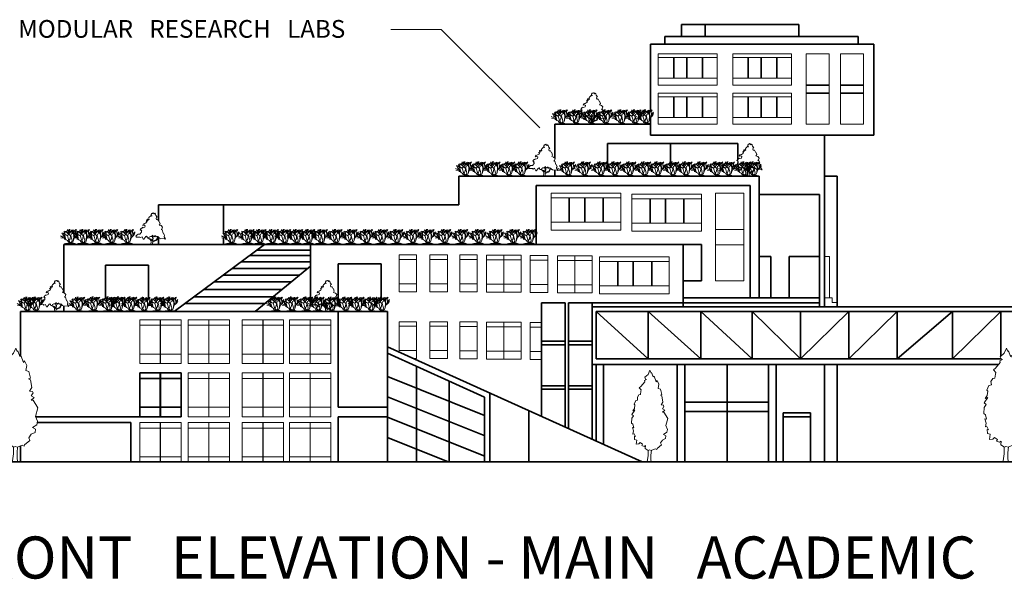
# Model space of a CAD drawing. Units: inches. Extents: x -1080 to 1950, y -1929 to 857.
# Tile 3 of 16: x -622 to -30, y -61 to 275. Entities that reach past the tile are written whole.
import ezdxf

# ---------------------------------------------------------------- set-up
doc = ezdxf.new("R2010")
doc.units = ezdxf.units.IN
doc.header["$MEASUREMENT"] = 0
for name, color, linetype, lineweight in [('A-ANNO-SYMB', 2, 'Continuous', 18), ('A-ANNO-TEXT', 7, 'Continuous', 25), ('A-ELEV', 7, 'Continuous', 35), ('A-GLAZ', 4, 'Continuous', 18), ('L-PLNT', 82, 'Continuous', 13)]:
    doc.layers.add(name, color=color, linetype=linetype, lineweight=lineweight)
doc.styles.get("Standard").update_dxf_attribs({"font": 'arial.ttf'})

# ---------------------------------------------------------------- blocks, each defined once
blk = doc.blocks.new('*U5')
blk.add_lwpolyline([(-2.754, 191.699), (-6.78, 182.851), (-13.682, 176.953), (-11.956, 173.266), (-9.656, 172.529), (-14.257, 170.317), (-13.682, 167.368), (-21.733, 157.783), (-25.184, 154.834), (-21.158, 150.41), (-21.733, 147.461), (-22.884, 140.825), (-26.334, 140.087), (-29.21, 134.926), (-28.635, 129.028), (-32.661, 128.291), (-36.111, 120.18), (-34.386, 118.706), (-35.536, 111.333), (-38.987, 106.171), (-34.386, 107.646), (-40.712, 98.798), (-37.261, 95.849), (-40.712, 90.688), (-41.287, 80.366), (-38.412, 78.154), (-36.686, 70.781), (-39.562, 71.518), (-37.261, 64.145), (-38.412, 57.509), (-36.111, 58.247), (-33.236, 52.348), (-35.536, 53.086), (-34.961, 46.45), (-30.36, 44.975), (-31.51, 36.128), (-26.334, 36.865), (-23.459, 39.814), (-18.283, 36.128), (-20.008, 33.178), (-14.832, 31.704), (-11.956, 33.178), (-12.531, 27.28), (-6.205, 22.856), (-3.905, 24.331), (0.121, 22.856), (8.173, 26.543), (11.624, 25.068), (12.199, 27.28), (21.4, 34.653), (19.675, 39.077), (23.701, 44.975), (30.027, 47.924), (30.602, 53.823), (25.426, 56.772), (32.903, 61.196), (34.053, 67.094), (30.602, 75.205), (34.628, 89.951), (26.576, 103.222), (23.701, 103.222), (28.302, 107.646), (23.701, 110.595), (26.576, 115.756), (25.426, 117.968), (20.825, 118.706), (24.276, 124.604), (22.551, 137.876), (19.1, 139.35), (22.551, 140.825), (19.675, 151.884), (14.499, 153.359), (16.224, 162.207), (12.199, 170.317), (10.473, 167.368), (5.872, 179.165), (4.147, 177.69), (0.696, 187.275), (-0.454, 185.8)], close=True)
for points in [[(-6.813, 23.669), (-6.813, 11.669), (-8.627, 0)], [(0.387, 23.669), (-0.576, 13.271), (-0.576, 3.686), (0, 0)]]:
    blk.add_lwpolyline(points)
blk = doc.blocks.new('*U2')
for points in [[(22.0124, 137.721), (18.5475, 141.5624), (15.5282, 138.2446), (13.8028, 139.3505), (13.3714, 142.1153), (11.2148, 143.2214), (8.1954, 140.4564), (4.7447, 141.0094), (2.1567, 136.0326), (2.1567, 131.6088), (5.6074, 129.9499), (3.0193, 128.2909), (0.4313, 130.5029), (-6.9015, 123.3141), (-6.9015, 121.6552), (-9.9208, 119.9963), (-9.0581, 118.3373), (-6.9015, 115.0195), (-10.7835, 112.2546), (-14.6656, 115.0195), (-16.8222, 114.4665), (-17.6849, 112.2546), (-14.6656, 111.7016), (-14.2342, 107.2778), (-17.6065, 107.8307), (-21.5669, 103.9599), (-17.2536, 103.4069), (-18.9789, 97.8771), (-22.8609, 97.3241), (-27.1743, 94.5593), (-32.3504, 91.7944), (-32.7817, 94.0063), (-36.6638, 85.7116), (-29.7624, 87.3705), (-25.449, 84.6056), (-26.743, 77.9699), (-34.507, 75.205), (-37.9578, 77.4169), (-39.2518, 74.099), (-42.2711, 73.5461), (-44.8592, 70.2282), (-47.8786, 66.3574), (-43.9965, 63.0395), (-41.4085, 64.6985), (-44.3346, 59.8898), (-42.2089, 60.1377), (-42.5159, 55.7849), (-49.6039, 46.4502), (-58.2307, 45.8972), (-62.1127, 43.6853), (-68.5828, 36.4966), (-65.9947, 32.0727), (-50.0352, 32.6257), (-47.0159, 30.4138), (-39.6831, 33.7317), (-34.507, 22.6721), (-32.3504, 22.6721), (-22.4296, 34.8376), (-19.4102, 36.4966), (-17.2536, 33.7317), (-17.2536, 29.8608), (-13.8028, 28.7549), (-9.0581, 28.7549), (-7.3328, 32.6257), (-1.7254, 35.3906), (3.8821, 35.9436), (6.4701, 38.1555), (6.9014, 38.7085), (8.1954, 41.4734), (9.9208, 40.3674), (11.2148, 35.9436), (14.2341, 37.6025), (15.0968, 36.4966), (15.9595, 33.7317), (18.9789, 38.7085), (21.9982, 38.7085), (23.2922, 36.4966), (21.9982, 34.2847), (25.4489, 35.3906), (26.743, 33.7317), (29.7623, 35.9436), (32.7817, 34.8376), (38.8204, 28.7549), (41.4084, 27.6489), (43.5651, 25.437), (61.6813, 27.0959), (65.132, 23.7781), (67.7201, 24.884), (60.8186, 33.7317), (60.3873, 37.0495), (62.544, 40.3674), (58.662, 50.874), (56.5053, 50.874), (52.1919, 66.3574), (47.8785, 66.9103), (50.4665, 69.1222), (53.9172, 77.9699), (47.0158, 85.1586), (38.3891, 87.9235), (42.2711, 94.0063)], [(42.2711, 94.0063), (38.8204, 104.5129), (36.6637, 104.5129), (32.3503, 113.9135), (29.7623, 113.3605), (26.743, 113.3605), (24.5862, 117.7844), (25.8802, 123.8671), (29.331, 123.8671), (22.8609, 131.6088), (21.9982, 137.6916)], [(-12.9401, 28.7549), (-2.588, 22.1191), (0.8626, 17.6953), (1.7253, 11.6125), (0, 0)], [(-9.9208, 28.2019), (0, 23.2251), (3.4507, 19.9072), (4.7447, 15.4834), (8.6267, 27.0959), (6.4701, 37.6025)], [(34.5071, 33.1787), (27.1743, 18.2483), (9.0581, 10.5066), (7.7641, 3.8708), (8.1954, 0)], [(8.1954, 40.3674), (11.2148, 27.6489), (8.1954, 13.8245), (24.5862, 19.9072), (32.7817, 34.2847)]]:
    blk.add_lwpolyline(points)
blk = doc.blocks.new('*U6')
for p, q in [((-463.296, 280.416), (-552.577, 423.037)), ((-329.184, 316.992), (-499.872, 414.528)), ((-426.72, 414.528), (-475.488, 475.488)), ((-377.952, 463.296), (-451.104, 487.68)), ((-426.72, 414.528), (-390.144, 499.872)), ((-426.72, 316.992), (-426.72, 414.528)), ((-377.952, 463.296), (-329.184, 524.256)), ((-207.264, 304.8), (-377.952, 463.296)), ((-338.455, 424.7896), (-290.3982, 464.5406)), ((-329.184, 316.992), (-207.264, 451.104)), ((-316.7634, 502.285), (-327.6092, 559.9176)), ((-296.5958, 484.4034), (-316.7634, 502.285)), ((-286.512, 498.3226), (-307.4416, 538.0736)), ((-305.8922, 396.9512), (-302.7934, 478.4344)), ((-304.3428, 426.7708), (-268.7066, 458.5716)), ((-302.7934, 478.4344), (-270.256, 518.1854)), ((-290.3982, 464.5406), (-265.6078, 577.8246)), ((-268.7066, 458.5716), (-250.0884, 500.3038)), ((-207.264, 451.104), (-268.224, 548.64)), ((-240.792, 502.285), (-228.3968, 573.8368)), ((-182.88, 499.872), (-219.456, 512.064)), ((-207.264, 451.104), (-134.112, 487.68)), ((-182.88, 499.872), (-158.496, 536.448)), ((-121.92, 414.528), (-182.88, 499.872)), ((-182.88, 377.952), (-97.536, 426.72)), ((-129.1844, 450.6214), (-140.0302, 542.036)), ((-134.112, 487.68), (-97.536, 548.64)), ((-85.7758, 389.001), (-129.1844, 452.6026)), ((-73.152, 329.184), (-109.728, 499.872)), ((-97.536, 426.72), (-24.384, 524.256)), ((-85.7758, 472.4908), (-73.3552, 548.005)), ((-70.2564, 426.7708), (-85.7758, 472.4908)), ((-73.152, 402.336), (-60.96, 512.064)), ((-24.384, 268.224), (-73.152, 402.336)), ((-12.9032, 555.9552), (-2.0574, 522.1732)), ((-5.1562, 486.3846), (2.5908, 542.036)), ((8.7884, 335.3562), (-5.1562, 486.3846)), ((-3.6068, 492.3536), (14.986, 518.1854)), ((-0.508, 508.254), (22.7584, 536.067)), ((1.0414, 526.1356), (35.1536, 559.9176)), ((2.5908, 542.036), (21.209, 555.9552)), ((8.7884, 335.3562), (33.6042, 412.8516)), ((24.384, 304.8), (36.576, 390.144)), ((33.6042, 412.8516), (92.5068, 464.5406)), ((36.576, 390.144), (73.152, 438.912)), ((48.768, 341.376), (60.96, 390.144)), ((60.96, 390.144), (85.344, 414.528)), ((-451.104, 219.456), (-601.0402, 303.8094)), ((-451.104, 219.456), (-587.4512, 234.2388)), ((-463.296, 280.416), (-512.064, 292.608)), ((-353.568, 316.992), (-487.68, 377.952)), ((-402.336, 207.264), (-463.296, 280.416)), ((-414.528, 182.88), (-463.296, 182.88)), ((-426.72, 316.992), (-451.104, 329.184)), ((-377.952, 146.304), (-451.104, 219.456)), ((-402.336, 12.192), (-451.104, 0)), ((-402.336, 207.264), (-426.72, 316.992)), ((-377.952, 146.304), (-402.336, 207.264)), ((-341.376, 12.192), (-402.336, 12.192)), ((-329.184, 121.92), (-377.952, 146.304)), ((-329.184, 316.992), (-353.568, 316.992)), ((-243.84, 24.384), (-341.376, 12.192)), ((-268.224, 109.728), (-329.184, 316.992)), ((-292.608, 60.96), (-329.184, 121.92)), ((-243.84, 24.384), (-329.184, 0)), ((-219.456, 24.384), (-292.608, 60.96)), ((-268.224, 109.728), (-219.456, 195.072)), ((-219.456, 48.768), (-268.224, 109.728)), ((-243.84, 24.384), (-195.072, 24.384)), ((-219.456, 195.072), (-207.264, 304.8)), ((-219.456, 24.384), (-109.728, 73.152)), ((-219.456, 24.384), (-158.496, 73.152)), ((-219.456, 24.384), (-219.456, 48.768)), ((-219.456, 24.384), (-73.152, 24.384)), ((-195.072, 316.992), (-182.88, 377.952)), ((-170.688, 219.456), (-195.072, 316.992)), ((-195.072, 24.384), (-158.496, 12.192)), ((-146.304, 134.112), (-170.688, 219.456)), ((-158.496, 73.152), (-146.304, 134.112)), ((-158.496, 12.192), (-85.344, 0)), ((-109.728, 73.152), (-48.768, 243.84)), ((-85.344, 134.112), (-73.152, 329.184)), ((-73.152, 24.384), (0, 0)), ((-48.768, 243.84), (24.384, 304.8)), ((-12.192, 274.32), (8.7884, 335.3562)), ((24.384, 304.8), (73.152, 377.952))]:
    blk.add_line(p, q)
blk = doc.blocks.new('*U4')
for points in [[(559.11496, 3498.1134), (471.1065, 3595.68496), (394.41628, 3511.41284), (350.59112, 3539.5027), (339.63356, 3609.72862), (284.85592, 3637.82356), (208.16316, 3567.59256), (120.51538, 3581.63876), (54.78018, 3455.22804), (54.78018, 3342.86352), (142.42796, 3300.72746), (76.69022, 3258.58886), (10.95502, 3314.77366), (-175.2981, 3132.17814), (-175.2981, 3090.04208), (-251.98832, 3047.90602), (-230.07574, 3005.76742), (-175.2981, 2921.4953), (-273.9009, 2851.26684), (-372.50624, 2921.4953), (-427.28388, 2907.4491), (-449.19646, 2851.26684), (-372.50624, 2837.22064), (-361.54868, 2724.85612), (-447.2051, 2738.89978), (-547.79926, 2640.58146), (-438.24144, 2626.53526), (-482.06406, 2486.07834), (-580.66686, 2472.03214), (-690.22722, 2401.80622), (-821.70016, 2331.57776), (-832.65518, 2387.76002), (-931.26052, 2177.07464), (-755.96496, 2219.2107), (-646.4046, 2148.98224), (-679.2722, 1980.43546), (-876.4778, 1910.207), (-964.12812, 1966.38926), (-996.99572, 1882.1146), (-1073.68594, 1868.07094), (-1139.42368, 1783.79628), (-1216.11644, 1685.47796), (-1117.5111, 1601.2033), (-1051.7759, 1643.3419), (-1126.09884, 1521.20092), (-1072.10606, 1527.49758), (-1079.90386, 1416.93646), (-1259.93906, 1179.83508), (-1479.05978, 1165.78888), (-1577.66258, 1109.60662), (-1742.00312, 927.01364), (-1676.26538, 814.64658), (-1270.89408, 828.69278), (-1194.20386, 772.51052), (-1007.95074, 856.78518), (-876.4778, 575.87134), (-821.70016, 575.87134), (-569.71184, 884.87504), (-493.01908, 927.01364), (-438.24144, 856.78518), (-438.24144, 758.46432), (-350.59112, 730.37446), (-230.07574, 730.37446), (-186.25312, 828.69278), (-43.82516, 898.92124), (98.60534, 912.96744), (164.34054, 969.1497), (175.29556, 983.1959), (208.16316, 1053.42436), (251.98832, 1025.33196), (284.85592, 912.96744), (361.54614, 955.1035), (383.45872, 927.01364), (405.3713, 856.78518), (482.06406, 983.1959), (558.75428, 983.1959), (591.62188, 927.01364), (558.75428, 870.83138), (646.40206, 898.92124), (679.2722, 856.78518), (755.96242, 912.96744), (832.65518, 884.87504), (986.03816, 730.37446), (1051.77336, 702.28206), (1106.55354, 646.0998), (1566.70502, 688.23586), (1654.3528, 603.96374), (1720.09054, 632.0536), (1544.79244, 856.78518), (1533.83742, 941.0573), (1588.6176, 1025.33196), (1490.0148, 1292.1996), (1435.23462, 1292.1996), (1325.67426, 1685.47796), (1216.1139, 1699.52162), (1281.8491, 1755.70388), (1369.49688, 1980.43546), (1194.20132, 2163.02844), (975.08314, 2233.2569), (1073.68594, 2387.76002)], [(1073.68594, 2387.76002), (986.03816, 2654.62766), (931.25798, 2654.62766), (821.69762, 2893.4029), (755.96242, 2879.3567), (679.2722, 2879.3567), (624.48948, 2991.72376), (657.35708, 3146.22434), (745.0074, 3146.22434), (580.66686, 3342.86352), (558.75428, 3497.36664)], [(-328.67854, 730.37446), (-65.7352, 561.82514), (21.91004, 449.46062), (43.82262, 294.9575), (0, 0)], [(-251.98832, 716.32826), (0, 589.91754), (87.64778, 505.64288), (120.51538, 393.27836), (219.11818, 688.23586), (164.34054, 955.1035)], [(876.48034, 842.73898), (690.22722, 463.50682), (230.07574, 266.86764), (197.20814, 98.31832), (208.16316, 0)], [(208.16316, 1025.33196), (284.85592, 702.28206), (208.16316, 351.1423), (624.48948, 505.64288), (832.65518, 870.83138)]]:
    blk.add_lwpolyline(points)
blk = doc.blocks.new('WIN-TYPE-A')
for p, q in [((12.45, 26.32), (0, 26.32)), ((0, 26.32), (0, 23.06)), ((24.78, 26.32), (12.34, 26.32)), ((12.34, 26.32), (12.34, 23.06)), ((12.45, 26.32), (12.45, 23.06)), ((24.78, 26.32), (24.78, 23.06)), ((0, 23.06), (0, 5.73)), ((0, 23.06), (12.45, 23.06)), ((12.34, 23.06), (12.34, 5.73)), ((12.34, 23.06), (24.78, 23.06)), ((12.45, 5.73), (12.45, 23.06)), ((24.78, 5.73), (24.78, 23.06)), ((0, 5.73), (12.45, 5.73)), ((0, 5.73), (0, 0)), ((0, 0), (12.45, 0)), ((12.34, 5.73), (24.78, 5.73)), ((12.34, 5.73), (12.34, 0)), ((12.34, 0), (24.78, 0)), ((12.45, 0), (12.45, 5.73)), ((24.78, 0), (24.78, 5.73))]:
    blk.add_line(p, q)
blk = doc.blocks.new('WIN-TYPE-B')
for p, q in [((10.5, 22.21), (0, 22.21)), ((0, 22.21), (0, 19.45)), ((0, 19.45), (0, 4.84)), ((0, 19.45), (10.5, 19.45)), ((20.91, 22.21), (10.41, 22.21)), ((10.41, 22.21), (10.41, 19.45)), ((10.41, 19.45), (10.41, 4.84)), ((10.41, 19.45), (20.91, 19.45)), ((10.5, 22.21), (10.5, 19.45)), ((10.5, 4.84), (10.5, 19.45)), ((20.91, 22.21), (20.91, 19.45)), ((20.91, 4.84), (20.91, 19.45)), ((0, 4.84), (10.5, 4.84)), ((0, 4.84), (0, 0)), ((0, 0), (10.5, 0)), ((10.41, 4.84), (20.91, 4.84)), ((10.41, 4.84), (10.41, 0)), ((10.41, 0), (20.91, 0)), ((10.5, 0), (10.5, 4.84)), ((20.91, 0), (20.91, 4.84))]:
    blk.add_line(p, q)
blk = doc.blocks.new('WIN-TYPE-C')
for p, q in [((12.45, 23.64), (0, 23.64)), ((0, 23.64), (0, 20.37)), ((0, 20.37), (0, 3.04)), ((0, 20.37), (12.45, 20.37)), ((24.78, 23.64), (12.34, 23.64)), ((12.34, 23.64), (12.34, 20.37)), ((12.34, 20.37), (12.34, 3.04)), ((12.34, 20.37), (24.78, 20.37)), ((12.45, 23.64), (12.45, 20.37)), ((12.45, 3.04), (12.45, 20.37)), ((24.78, 23.64), (24.78, 20.37)), ((24.78, 3.04), (24.78, 20.37)), ((0, 3.04), (12.45, 3.04)), ((0, 3.04), (0, 0)), ((12.34, 3.04), (24.78, 3.04)), ((12.34, 3.04), (12.34, 0)), ((12.45, 0), (12.45, 3.04)), ((24.78, 0), (24.78, 3.04))]:
    blk.add_line(p, q)
blk = doc.blocks.new('WIN-TYPE-E')
for p, q in [((10.5, 22.21), (0, 22.21)), ((0, 22.21), (0, 19.45)), ((0, 19.45), (0, 4.84)), ((0, 19.45), (10.5, 19.45)), ((10.5, 22.21), (10.5, 19.45)), ((10.5, 4.84), (10.5, 19.45)), ((0, 4.84), (10.5, 4.84)), ((0, 4.84), (0, 0)), ((0, 0), (10.5, 0)), ((10.5, 0), (10.5, 4.84))]:
    blk.add_line(p, q)
blk = doc.blocks.new('WIN-TYPE-G')
for p, q in [((0, 19.45), (0, 22.21)), ((0, 22.21), (41.85, 22.21)), ((0, 19.45), (0, 4.84)), ((41.85, 19.45), (0, 19.45)), ((41.85, 22.21), (41.85, 19.45)), ((41.85, 4.84), (41.85, 19.45)), ((0, 4.84), (41.85, 4.84)), ((0, 4.84), (0, 0)), ((41.85, 0), (41.85, 4.84)), ((0, 0), (41.85, 0))]:
    blk.add_line(p, q)
blk = doc.blocks.new('WIN-TYPE-H')
for p, q in [((0, 16.47), (0, 18.8)), ((0, 18.8), (35.42, 18.8)), ((35.42, 18.8), (35.42, 16.47)), ((0, 16.47), (0, 4.09)), ((35.42, 16.47), (0, 16.47)), ((35.42, 4.09), (35.42, 16.47)), ((0, 4.09), (35.42, 4.09)), ((0, 4.09), (0, 0)), ((35.42, 0), (35.42, 4.09)), ((0, 0), (35.42, 0))]:
    blk.add_line(p, q)
blk = doc.blocks.new('WIN-TYPE-N')
for p, q in [((0, 52.66), (17.07, 52.66)), ((0, 30.88), (0, 52.66)), ((17.07, 52.66), (17.07, 30.88)), ((17.07, 30.88), (0, 30.88)), ((0, 30.88), (0, 21.78)), ((17.07, 30.88), (17.07, 21.78)), ((0, 21.78), (17.07, 21.78)), ((0, 0), (0, 21.78)), ((17.07, 21.78), (17.07, 0)), ((17.07, 0), (0, 0))]:
    blk.add_line(p, q)
blk = doc.blocks.new('WIN-TYPE-P')
for p, q in [((10.5, 22.21), (0, 22.21)), ((0, 22.21), (0, 19.45)), ((0, 19.45), (0, 4.84)), ((0, 19.45), (10.5, 19.45)), ((10.5, 22.21), (10.5, 19.45)), ((10.5, 4.84), (10.5, 19.45)), ((0, 4.84), (10.5, 4.84)), ((0, 4.84), (0, 3.89)), ((8.62, 0), (10.5, 0)), ((10.5, 0), (10.5, 4.84))]:
    blk.add_line(p, q)
blk = doc.blocks.new('PANEL-A')
for p, q in [((0, 42.42), (0, 0)), ((13.76, 42.42), (0, 42.42)), ((13.76, 0), (13.76, 42.42)), ((0, 0), (13.76, 0))]:
    blk.add_line(p, q)
blk = doc.blocks.new('WIN-TYPE-R')
for p, q in [((6.66, 22.21), (0, 22.21)), ((0, 22.21), (0, 19.45)), ((0, 19.45), (0, 4.84)), ((0, 19.45), (6.66, 19.45)), ((0, 4.84), (6.66, 4.84)), ((0, 4.84), (0, 0)), ((0, 0), (6.66, 0))]:
    blk.add_line(p, q)
blk = doc.blocks.new('WIN-TYPE-S')
for p, q in [((0, 27.66), (3.06, 27.66)), ((3.06, 27.66), (3.06, 2.78)), ((3.06, 2.78), (0, 2.78)), ((3.06, 2.78), (4.6, 2.78)), ((4.6, 2.78), (4.6, 0)), ((4.6, 0), (7.75, 0))]:
    blk.add_line(p, q)

msp = doc.modelspace()

# ---------------------------------------------------------------- linework, layer by layer
at = {"layer": 'A-ANNO-SYMB'}
for q in [(-398.58, 268.75), (-308.98, 209.71)]:
    msp.add_line((-368.35, 268.75), q, dxfattribs=at)
at = {"layer": 'A-ELEV'}
for p, q in [((-223.9, 269.6), (-223.9, 271.66)), ((-223.9, 271.66), (-153.32, 271.66)), ((-223.9, 264.54), (-223.9, 269.6)), ((-209.57, 264.54), (-209.57, 271.66)), ((-153.32, 271.66), (-153.32, 264.54)), ((-233.84, 260.04), (-233.84, 264.54)), ((-233.84, 264.54), (-117.77, 264.54)), ((-117.77, 264.54), (-117.77, 260.04)), ((-242.4, 250.46), (-242.4, 260.04)), ((-242.4, 260.04), (-112.68, 260.04)), ((-112.68, 260.04), (-108.18, 260.04)), ((-108.18, 260.04), (-108.18, 210.83)), ((-242.4, 234.12), (-242.4, 250.46)), ((-228.5, 251.89), (-228.5, 239.51)), ((-220.66, 251.89), (-220.66, 239.51)), ((-211.25, 251.89), (-211.25, 239.51)), ((-183.82, 251.89), (-183.82, 239.51)), ((-175.98, 251.89), (-175.98, 239.51)), ((-166.57, 251.89), (-166.57, 239.51)), ((-242.4, 234.12), (-242.4, 219.88)), ((-148.84, 235.42), (-135.08, 235.42)), ((-128.29, 235.42), (-114.53, 235.42)), ((-228.5, 228.27), (-228.5, 215.89)), ((-220.66, 228.27), (-220.66, 215.89)), ((-211.25, 228.27), (-211.25, 215.89)), ((-183.82, 228.27), (-183.82, 215.89)), ((-175.98, 228.27), (-175.98, 215.89)), ((-166.57, 228.27), (-166.57, 215.89)), ((-148.84, 230.6), (-135.08, 230.6)), ((-128.29, 230.6), (-114.53, 230.6)), ((-242.4, 216.14), (-242.4, 206.68)), ((-242.4, 211.8), (-299.96, 211.8)), ((-299.96, 211.8), (-299.96, 191.39)), ((-108.18, 205.21), (-108.18, 210.83)), ((-242.4, 205.21), (-242.4, 206.68)), ((-144.09, 205.21), (-242.4, 205.21)), ((-144.09, 205.21), (-108.18, 205.21)), ((-137.95, 205.21), (-137.95, 102.28)), ((-268.41, 187.18), (-268.41, 200.27)), ((-268.41, 200.27), (-190.05, 200.27)), ((-230.41, 200.27), (-230.41, 186.07)), ((-190.05, 200.27), (-190.05, 190.71)), ((-299.96, 184.41), (-299.96, 180.63)), ((-268.41, 184.1), (-268.41, 185.92)), ((-357.6, 180.63), (-357.6, 163.4)), ((-177.27, 180.63), (-357.6, 180.63)), ((-230.41, 180.95), (-230.41, 180.63)), ((-189.87, 180.68), (-189.87, 180.63)), ((-177.27, 180.63), (-177.27, 107.59)), ((-137.95, 180.63), (-130.2, 180.63)), ((-130.2, 180.63), (-130.2, 102.28)), ((-182.61, 175.14), (-311.15, 175.14)), ((-311.15, 175.14), (-311.15, 146.63)), ((-182.61, 175.14), (-182.61, 107.59)), ((-291.28, 167.62), (-291.28, 153)), ((-282.01, 167.62), (-282.01, 153)), ((-270.9, 167.62), (-270.9, 153)), ((-242.75, 167.07), (-242.75, 152.45)), ((-233.49, 167.07), (-233.49, 152.45)), ((-222.38, 167.07), (-222.38, 152.45)), ((-177.27, 169.72), (-140.99, 169.72)), ((-140.99, 169.72), (-140.99, 102.28)), ((-538.13, 163.4), (-538.13, 153.85)), ((-499.1, 163.4), (-538.13, 163.4)), ((-357.6, 163.4), (-500.54, 163.4)), ((-499.1, 163.4), (-499.1, 145.94)), ((-499.1, 145.94), (-499.1, 163.4)), ((-538.13, 143.98), (-538.13, 139.7)), ((-538.13, 142.55), (-538.13, 140.7)), ((-499.1, 143.57), (-499.1, 139.7)), ((-499.1, 139.7), (-499.1, 143.57)), ((-311.15, 145.47), (-311.15, 139.7)), ((-311.15, 139.7), (-595.05, 139.7)), ((-595.05, 139.7), (-595.05, 110.56)), ((-474.45, 139.7), (-528.73, 99.4)), ((-479.2, 136.17), (-446.74, 136.17)), ((-446.74, 104.8), (-446.74, 139.7)), ((-222.88, 139.7), (-311.15, 139.7)), ((-222.88, 107.59), (-222.88, 139.7)), ((-222.88, 139.7), (-211.87, 139.7)), ((-211.87, 139.7), (-211.87, 117.73)), ((-483.5, 132.98), (-446.74, 132.98)), ((-170.17, 132.47), (-177.27, 132.47)), ((-170.17, 132.47), (-170.17, 107.59)), ((-140.99, 132.47), (-159.06, 132.47)), ((-159.06, 132.47), (-159.06, 107.59)), ((-544.08, 127.31), (-569.96, 127.31)), ((-569.96, 127.31), (-569.96, 107.83)), ((-544.08, 107.26), (-544.08, 127.31)), ((-493.85, 125.3), (-448.32, 125.3)), ((-488.44, 129.31), (-446.74, 129.31)), ((-446.74, 126.59), (-480.05, 99.4)), ((-404.41, 127.96), (-430.29, 127.96)), ((-430.29, 127.96), (-430.29, 105.94)), ((-404.41, 127.96), (-404.41, 105.75)), ((-262.14, 129.43), (-262.14, 114.82)), ((-252.87, 129.43), (-252.87, 114.82)), ((-241.76, 129.43), (-241.76, 114.82)), ((-499.47, 121.13), (-453.43, 121.13)), ((-510.93, 112.62), (-463.85, 112.62)), ((-504.84, 117.14), (-458.32, 117.14)), ((-211.87, 117.73), (-222.88, 117.73)), ((-516.9, 108.19), (-469.28, 108.19)), ((-182.61, 107.59), (-222.88, 107.59)), ((-222.88, 107.59), (-222.88, 102.28)), ((-222.88, 107.59), (-140.99, 107.59)), ((-595.05, 102.6), (-595.05, 99.4)), ((-569.96, 106.21), (-569.96, 105.86)), ((-569.96, 104.47), (-569.96, 104.15)), ((-544.08, 103.03), (-544.08, 103.83)), ((-522.4, 104.1), (-474.29, 104.1)), ((-308.06, 104.57), (-308.06, 102.28)), ((-293.75, 104.57), (-308.06, 104.57)), ((-308.06, 102.28), (-308.06, 36.38)), ((-293.75, 29.92), (-293.75, 104.57)), ((-222.88, 104.57), (-291.77, 104.57)), ((-291.77, 29.03), (-291.77, 104.57)), ((-277.64, 22.66), (-277.64, 104.57)), ((-222.88, 102.28), (-277.64, 102.28)), ((-222.88, 104.57), (-140.99, 104.57)), ((-222.88, 102.28), (-137.95, 102.28)), ((-123.32, 102.28), (-177.27, 102.28)), ((-123.32, 102.28), (2.16, 102.28)), ((-621.1, 72.79), (-621.1, 99.4)), ((-621.1, 99.4), (-400.95, 99.4)), ((-544.08, 99.4), (-544.08, 99.5)), ((-446.74, 99.4), (-446.74, 99.82)), ((-430.29, 99.4), (-430.29, 41.92)), ((-400.48, 99.4), (-409.25, 99.4)), ((-404.41, 100.02), (-404.41, 99.85)), ((-400.48, 99.4), (-400.95, 99.4)), ((-400.48, 99.4), (-400.48, 9.02)), ((-222.88, 99.4), (-275.18, 99.4)), ((-275.18, 99.4), (-275.18, 70.95)), ((-275.18, 99.4), (-243.84, 70.95)), ((-243.84, 99.4), (-243.84, 70.95)), ((-243.84, 99.4), (-212.24, 70.95)), ((-126.4, 99.4), (-222.88, 99.4)), ((-212.24, 99.4), (-212.24, 70.95)), ((-212.24, 99.4), (-181.47, 70.95)), ((-181.47, 99.4), (-181.47, 70.95)), ((-181.47, 99.4), (-152.43, 70.95)), ((-152.43, 99.4), (-152.43, 70.95)), ((-123.32, 99.4), (-152.43, 70.95)), ((1.28, 99.4), (-126.4, 99.4)), ((-123.32, 99.4), (-123.32, 70.95)), ((-94.28, 99.4), (-123.32, 70.95)), ((-94.28, 99.4), (-94.28, 70.95)), ((-60.92, 99.4), (-94.28, 70.95)), ((-60.92, 99.4), (-60.92, 70.95)), ((-31.87, 99.4), (-60.92, 70.95)), ((-31.87, 99.4), (-31.87, 72.61)), ((-400.48, 78.07), (-247.42, 9.02)), ((-308.06, 81.48), (-293.75, 81.48)), ((-308.06, 79.29), (-293.75, 79.29)), ((-291.77, 81.48), (-277.64, 81.48)), ((-291.77, 79.29), (-277.64, 79.29)), ((-400.48, 74.27), (-342.32, 47.95)), ((-31.87, 71.12), (-31.87, 70.95)), ((-383.06, 66.39), (-383.06, 9.02)), ((-112.28, 67.56), (-277.64, 67.56)), ((-123.32, 70.95), (-275.18, 70.95)), ((-275.18, 67.56), (-275.18, 25.36)), ((-270.65, 67.56), (-270.65, 19.5)), ((-226.43, 67.56), (-226.43, 9.02)), ((-221.76, 67.56), (-221.76, 9.02)), ((-196.36, 67.56), (-196.36, 9.02)), ((-171.52, 67.56), (-171.52, 9.02)), ((-166.86, 67.56), (-166.86, 9.02)), ((-137.95, 67.56), (-137.95, 9.02)), ((-130.2, 67.56), (-130.2, 9.02)), ((-31.79, 70.95), (-123.32, 70.95)), ((-33.42, 67.56), (-112.28, 67.56)), ((-536.96, 62.51), (-549.41, 62.51)), ((-549.41, 62.51), (-549.41, 59.24)), ((-549.41, 59.24), (-549.41, 41.92)), ((-549.41, 59.24), (-536.96, 59.24)), ((-524.62, 62.51), (-537.07, 62.51)), ((-537.07, 62.51), (-537.07, 59.24)), ((-537.07, 59.24), (-537.07, 41.92)), ((-537.07, 59.24), (-524.62, 59.24)), ((-536.96, 62.51), (-536.96, 59.24)), ((-536.96, 41.92), (-536.96, 59.24)), ((-524.62, 62.51), (-524.62, 59.24)), ((-524.62, 41.92), (-524.62, 59.24)), ((-400.48, 60.25), (-342.32, 36.88)), ((-363.57, 57.57), (-363.57, 9.02)), ((-308.06, 54.7), (-293.75, 54.7)), ((-291.77, 54.7), (-277.64, 54.7)), ((-400.51, 48.23), (-342.36, 24.86)), ((-342.32, 51.98), (-342.32, 51.84)), ((-342.32, 47.95), (-342.32, 9.02)), ((-339.02, 50.35), (-339.02, 9.02)), ((-308.06, 52.64), (-293.75, 52.64)), ((-291.77, 52.64), (-277.64, 52.64)), ((-549.41, 41.92), (-536.96, 41.92)), ((-549.41, 41.92), (-549.41, 36.18)), ((-537.07, 41.92), (-524.62, 41.92)), ((-537.07, 41.92), (-537.07, 36.18)), ((-536.96, 36.18), (-536.96, 41.92)), ((-524.62, 36.18), (-524.62, 41.92)), ((-430.29, 41.92), (-400.48, 41.92)), ((-221.76, 44.86), (-171.52, 44.86)), ((-554.75, 36.18), (-612.12, 36.18)), ((-554.75, 36.18), (-549.41, 36.18)), ((-549.41, 36.18), (-536.96, 36.18)), ((-537.07, 36.18), (-524.62, 36.18)), ((-430.29, 36.18), (-400.48, 36.18)), ((-430.29, 36.18), (-430.29, 9.02)), ((-400.48, 35.85), (-342.68, 12.63)), ((-315.55, 39.76), (-315.55, 9.02)), ((-221.76, 39.31), (-171.52, 39.31)), ((-162.77, 38.54), (-146.32, 38.54)), ((-162.77, 38.54), (-162.77, 9.02)), ((-162.77, 36.1), (-146.32, 36.1)), ((-146.32, 38.54), (-146.32, 9.02)), ((-554.75, 32.66), (-611.1, 32.66)), ((-554.75, 32.66), (-554.75, 9.02)), ((-275.18, 25.36), (-275.18, 21.54)), ((-621.1, 9.02), (-621.1, 18.65)), ((-400.48, 23.63), (-364.13, 9.02)), ((-148.56, 9.02), (-740.58, 9.02)), ((-129.68, 9.02), (-740.58, 9.02)), ((709.45, 9.02), (-148.56, 9.02))]:
    msp.add_line(p, q, dxfattribs=at)

# ---------------------------------------------------------------- block references
at = {"layer": 'A-GLAZ'}
for name, p in [('WIN-TYPE-H', (-237.78, 235.42)), ('WIN-TYPE-H', (-193.1, 235.42)), ('PANEL-A', (-148.84, 211.8)), ('PANEL-A', (-128.29, 211.8)), ('WIN-TYPE-H', (-237.78, 211.8)), ('WIN-TYPE-H', (-193.1, 211.8)), ('WIN-TYPE-G', (-302.24, 148.16)), ('WIN-TYPE-G', (-253.72, 147.62)), ('WIN-TYPE-N', (-203.5, 117.73)), ('WIN-TYPE-E', (-393.56, 111.23)), ('WIN-TYPE-E', (-375.07, 111.23)), ('WIN-TYPE-E', (-357.11, 111.23)), ('WIN-TYPE-B', (-341.03, 110.95)), ('WIN-TYPE-E', (-314.72, 110.83)), ('WIN-TYPE-B', (-298.42, 110.64)), ('WIN-TYPE-G', (-273.1, 109.98)), ('WIN-TYPE-S', (-137.95, 104.81)), ('WIN-TYPE-A', (-549.41, 68.08)), ('WIN-TYPE-A', (-520.29, 68.08)), ('WIN-TYPE-A', (-487.79, 68.08)), ('WIN-TYPE-A', (-459.37, 68.08)), ('WIN-TYPE-P', (-393.56, 71.06)), ('WIN-TYPE-E', (-375.07, 71.06)), ('WIN-TYPE-E', (-357.11, 71.02)), ('WIN-TYPE-B', (-341.03, 70.74)), ('WIN-TYPE-R', (-314.72, 70.62)), ('WIN-TYPE-A', (-520.29, 36.18)), ('WIN-TYPE-A', (-487.79, 36.18)), ('WIN-TYPE-A', (-459.37, 36.18)), ('WIN-TYPE-C', (-549.41, 9.02)), ('WIN-TYPE-C', (-520.29, 9.02)), ('WIN-TYPE-C', (-487.79, 9.02)), ('WIN-TYPE-C', (-459.37, 9.02))]:
    msp.add_blockref(name, p, dxfattribs=at)
at = {"layer": 'L-PLNT'}
for name, p, xscale, yscale, zscale in [('*U2', (-278.15, 211.96), 0.1315554675521508, 0.1315554675521508, 0.1315554675521508), ('*U6', (-292.95, 211.95), 0.0152219259934872, 0.0152219259934872, 0.0152219259934872), ('*U6', (-284.2, 211.95), 0.0152219259934872, 0.0152219259934872, 0.0152219259934872), ('*U6', (-275.1, 211.95), 0.0152219259934872, 0.0152219259934872, 0.0152219259934872), ('*U6', (-266.24, 211.95), 0.0152219259934872, 0.0152219259934872, 0.0152219259934872), ('*U6', (-256.84, 211.95), 0.0152219259934872, 0.0152219259934872, 0.0152219259934872), ('*U6', (-248.63, 211.95), 0.0152219259934872, 0.0152219259934872, 0.0152219259934872), ('*U6', (-241.99, 211.95), 0.0152219259934872, 0.0152219259934872, 0.0152219259934872), ('*U2', (-306.88, 180.96), 0.1315554675521508, 0.1315554675521508, 0.1315554675521508), ('*U4', (-184.25, 181.23), 0.0052143573184964, 0.0052143573184964, 0.0052143573184964), ('*U6', (-350.59, 180.68), 0.0152219259934872, 0.0152219259934872, 0.0152219259934872), ('*U6', (-342.19, 180.68), 0.0152219259934872, 0.0152219259934872, 0.0152219259934872), ('*U6', (-333.42, 180.68), 0.0152219259934872, 0.0152219259934872, 0.0152219259934872), ('*U6', (-324.48, 180.68), 0.0152219259934872, 0.0152219259934872, 0.0152219259934872), ('*U6', (-316.75, 180.68), 0.0152219259934872, 0.0152219259934872, 0.0152219259934872), ('*U6', (-288.79, 180.68), 0.0152219259934872, 0.0152219259934872, 0.0152219259934872), ('*U6', (-279.02, 180.68), 0.0152219259934872, 0.0152219259934872, 0.0152219259934872), ('*U6', (-269.17, 180.68), 0.0152219259934872, 0.0152219259934872, 0.0152219259934872), ('*U6', (-260.78, 180.68), 0.0152219259934872, 0.0152219259934872, 0.0152219259934872), ('*U6', (-251.74, 180.68), 0.0152219259934872, 0.0152219259934872, 0.0152219259934872), ('*U6', (-242.85, 180.68), 0.0152219259934872, 0.0152219259934872, 0.0152219259934872), ('*U6', (-234.94, 180.68), 0.0152219259934872, 0.0152219259934872, 0.0152219259934872), ('*U6', (-225.91, 180.68), 0.0152219259934872, 0.0152219259934872, 0.0152219259934872), ('*U6', (-218.01, 180.68), 0.0152219259934872, 0.0152219259934872, 0.0152219259934872), ('*U6', (-209.11, 180.68), 0.0152219259934872, 0.0152219259934872, 0.0152219259934872), ('*U6', (-199.51, 180.68), 0.0152219259934872, 0.0152219259934872, 0.0152219259934872), ('*U6', (-192.46, 180.68), 0.0152219259934872, 0.0152219259934872, 0.0152219259934872), ('*U6', (-183, 180.68), 0.0152219259934872, 0.0152219259934872, 0.0152219259934872), ('*U6', (-177.31, 180.68), 0.0152219259934872, 0.0152219259934872, 0.0152219259934872), ('*U2', (-542.8, 139.76), 0.1315554675521508, 0.1315554675521508, 0.1315554675521508), ('*U6', (-587.9, 140.11), 0.0152219259934872, 0.0152219259934872, 0.0152219259934872), ('*U6', (-580.25, 140.11), 0.0152219259934872, 0.0152219259934872, 0.0152219259934872), ('*U6', (-572.01, 140.11), 0.0152219259934872, 0.0152219259934872, 0.0152219259934872), ('*U6', (-563.16, 140.11), 0.0152219259934872, 0.0152219259934872, 0.0152219259934872), ('*U6', (-553.68, 140.11), 0.0152219259934872, 0.0152219259934872, 0.0152219259934872), ('*U6', (-491.07, 140.11), 0.0152219259934872, 0.0152219259934872, 0.0152219259934872), ('*U6', (-481.15, 140.11), 0.0152219259934872, 0.0152219259934872, 0.0152219259934872), ('*U6', (-474.04, 140.11), 0.0152219259934872, 0.0152219259934872, 0.0152219259934872), ('*U6', (-466.5, 140.11), 0.0152219259934872, 0.0152219259934872, 0.0152219259934872), ('*U6', (-459.23, 140.11), 0.0152219259934872, 0.0152219259934872, 0.0152219259934872), ('*U6', (-451.98, 140.11), 0.0152219259934872, 0.0152219259934872, 0.0152219259934872), ('*U6', (-444.73, 140.11), 0.0152219259934872, 0.0152219259934872, 0.0152219259934872), ('*U6', (-437.21, 140.11), 0.0152219259934872, 0.0152219259934872, 0.0152219259934872), ('*U6', (-428.34, 140.11), 0.0152219259934872, 0.0152219259934872, 0.0152219259934872), ('*U6', (-419.32, 140.11), 0.0152219259934872, 0.0152219259934872, 0.0152219259934872), ('*U6', (-410, 140.11), 0.0152219259934872, 0.0152219259934872, 0.0152219259934872), ('*U6', (-400.89, 140.11), 0.0152219259934872, 0.0152219259934872, 0.0152219259934872), ('*U6', (-391.81, 140.11), 0.0152219259934872, 0.0152219259934872, 0.0152219259934872), ('*U6', (-382.17, 140.11), 0.0152219259934872, 0.0152219259934872, 0.0152219259934872), ('*U6', (-373.09, 140.11), 0.0152219259934872, 0.0152219259934872, 0.0152219259934872), ('*U6', (-363.01, 140.11), 0.0152219259934872, 0.0152219259934872, 0.0152219259934872), ('*U6', (-352.8, 140.11), 0.0152219259934872, 0.0152219259934872, 0.0152219259934872), ('*U6', (-342.58, 140.11), 0.0152219259934872, 0.0152219259934872, 0.0152219259934872), ('*U6', (-332.22, 140.11), 0.0152219259934872, 0.0152219259934872, 0.0152219259934872), ('*U6', (-321.76, 140.11), 0.0152219259934872, 0.0152219259934872, 0.0152219259934872), ('*U6', (-311.93, 140.11), 0.0152219259934872, 0.0152219259934872, 0.0152219259934872), ('*U2', (-600.88, 99.24), 0.1315554675521508, 0.1315554675521508, 0.1315554675521508), ('*U2', (-438.06, 99.24), 0.1315554675521508, 0.1315554675521508, 0.1315554675521508), ('*U6', (-613.89, 99.47), 0.0152219259934872, 0.0152219259934872, 0.0152219259934872), ('*U6', (-608.65, 99.47), 0.0152219259934872, 0.0152219259934872, 0.0152219259934872), ('*U6', (-583, 99.47), 0.0152219259934872, 0.0152219259934872, 0.0152219259934872), ('*U6', (-574.01, 99.57), 0.0152219259934872, 0.0152219259934872, 0.0152219259934872), ('*U6', (-565.02, 99.57), 0.0152219259934872, 0.0152219259934872, 0.0152219259934872), ('*U6', (-558.73, 99.57), 0.0152219259934872, 0.0152219259934872, 0.0152219259934872), ('*U6', (-551.66, 99.57), 0.0152219259934872, 0.0152219259934872, 0.0152219259934872), ('*U6', (-543.65, 99.35), 0.0152219259934872, 0.0152219259934872, 0.0152219259934872), ('*U6', (-535.45, 99.5), 0.0152219259934872, 0.0152219259934872, 0.0152219259934872), ('*U6', (-527.94, 99.5), 0.0152219259934872, 0.0152219259934872, 0.0152219259934872), ('*U6', (-464.17, 99.55), 0.0152219259934872, 0.0152219259934872, 0.0152219259934872), ('*U6', (-454.86, 99.55), 0.0152219259934872, 0.0152219259934872, 0.0152219259934872), ('*U6', (-445.93, 99.55), 0.0152219259934872, 0.0152219259934872, 0.0152219259934872), ('*U6', (-439.07, 99.55), 0.0152219259934872, 0.0152219259934872, 0.0152219259934872), ('*U6', (-431.01, 99.47), 0.0152219259934872, 0.0152219259934872, 0.0152219259934872), ('*U6', (-422.5, 99.47), 0.0152219259934872, 0.0152219259934872, 0.0152219259934872), ('*U6', (-415.08, 99.47), 0.0152219259934872, 0.0152219259934872, 0.0152219259934872), ('*U6', (-407.2, 99.47), 0.0152219259934872, 0.0152219259934872, 0.0152219259934872), ('*U6', (-400.71, 99.47), 0.0152219259934872, 0.0152219259934872, 0.0152219259934872), ('*U5', (-622.96, 9.75), 0.3528399638811642, 0.3528399638811642, 0.3528399638811642), ('*U5', (-27.54, 9.75), 0.3528399638811642, 0.3528399638811642, 0.3528399638811642), ('*U5', (-242.03, 9.33), 0.2857357741909547, 0.2857357741909547, 0.2857357741909547)]:
    msp.add_blockref(name, p, dxfattribs=dict(at, xscale=xscale, yscale=yscale, zscale=zscale))

# ---------------------------------------------------------------- texts
at = {"layer": 'A-ANNO-TEXT'}
for s, height, p in [('MODULAR   RESEARCH   LABS', 10.6643, (-622.54, 263.78)), ('FRONT   ELEVATION - MAIN   ACADEMIC   AND   INNOVATION   COMPLEX', 25.272, (-665.96, -61.01))]:
    msp.add_text(s, height=height, dxfattribs=at).set_placement(p)

doc.saveas('drawing.dxf')
